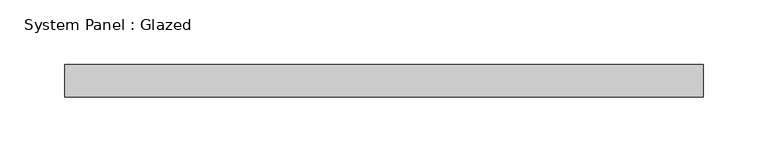
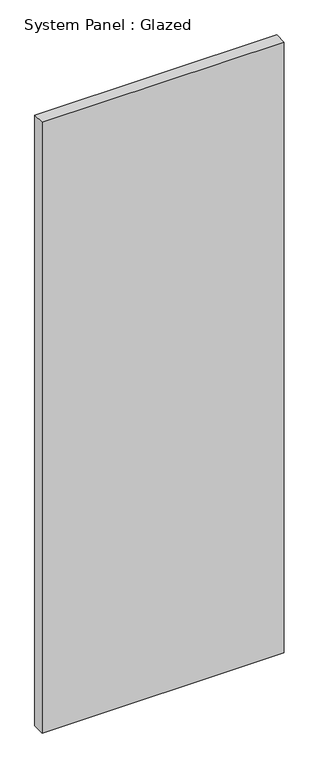
"""IFC4 building model written with IfcOpenShell, lengths in millimetres: plate geometry, System Panel : Glazed."""

from ifc_helpers import new_model, si_unit, origin, origin_with_axes, place, context, project, spatial, polyline, outline, extrude, source, transform, mapped, element, save


def system_panel_glazed_f8dc496e(model_context):
    return source(origin(), model_context, "Body", "SweptSolid", [
        extrude(outline(polyline([(247.65, 19.05), (-247.65, 19.05), (-247.65, 44.45), (247.65, 44.45), (247.65, 19.05)])), origin_with_axes(), (0.0, 0.0, 1.0), 1319.9422272),
    ])


if __name__ == "__main__":
    model = new_model("IFC4")
    model_context = context("Model", 3, world=origin())
    ifc_project = project(units=[si_unit("LENGTHUNIT", "METRE", prefix="MILLI")], contexts=[model_context])
    site = spatial("IfcSite", under=ifc_project)
    building = spatial("IfcBuilding", under=site)
    placement = place(None, origin())
    system_panel_glazed_shape = system_panel_glazed_f8dc496e(model_context)
    element("IfcPlate", 1, ObjectType="System Panel : Glazed", at=placement, inside=building, context=model_context, shape_type="MappedRepresentation", body=[
        mapped(system_panel_glazed_shape, transform((0.0, 0.0, 0.0), x_axis=(1.0, 0.0, 0.0), y_axis=(0.0, 1.0, 0.0), z_axis=(0.0, 0.0, 1.0))),
    ])
    save(model, "model.ifc")

# Revit data of these elements
# Type "System Panel : Glazed"
#   Construction Type Id = "GSP4R"
#   Analytic Construction = "1/8 in Pilkington single glazing"
#   Visual Light Transmittance = 0.9
#   Solar Heat Gain Coefficient = 0.86
#   Heat Transfer Coefficient (U) = 1.18115 BTU/(h·ft²·°F)
#   Define Thermal Properties by = 1
# Element 1 (IfcPlate, "System Panel : Glazed")
#   Materials on its faces: "Glass"
# Materials
#   "Glass": class "Glass", colour RGB 0 128 192, transparency 0.75, Description = "Soda Lime Glass", Cost = 0
